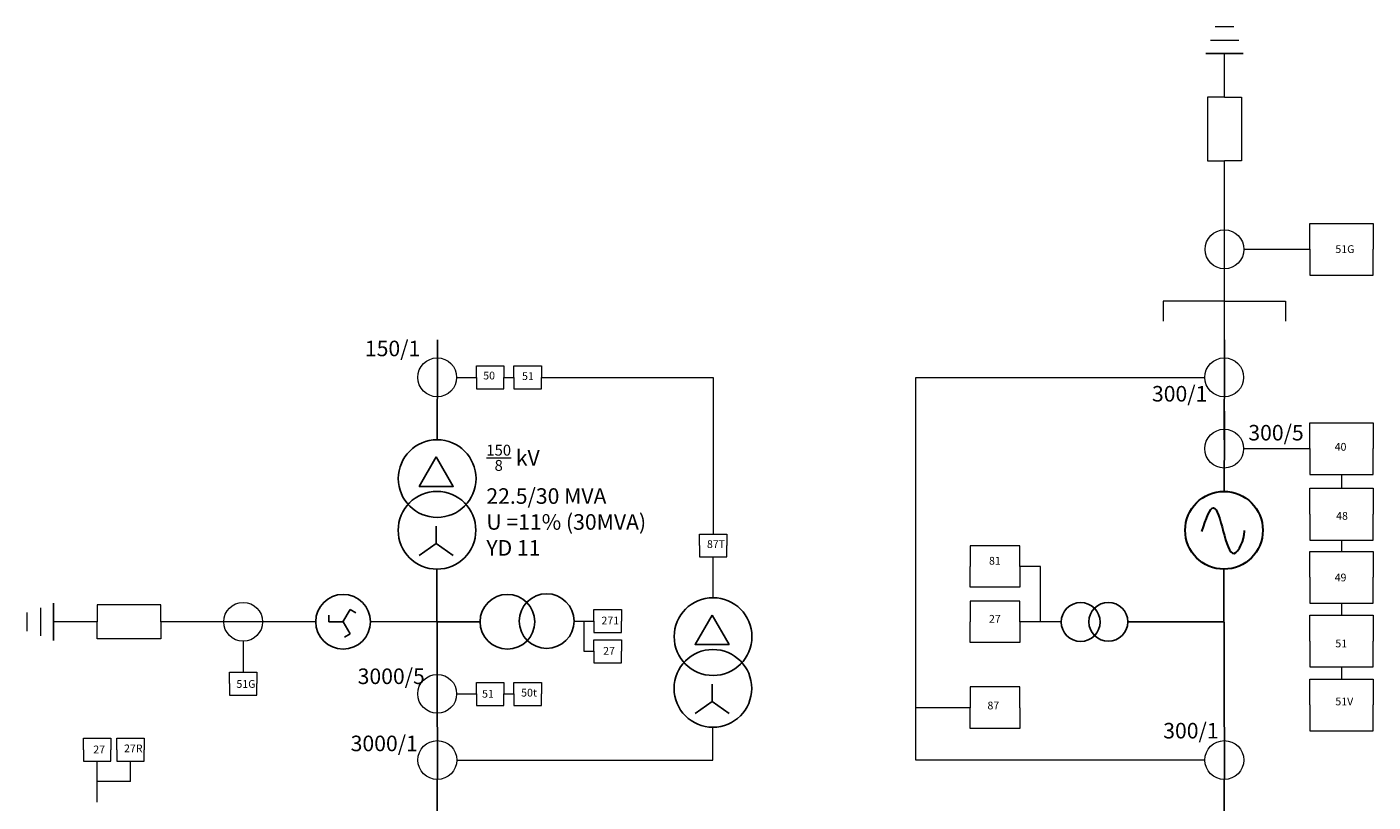
# Model space of a CAD drawing. Units: inches. Extents: x 77.1 to 95.7, y 45.4 to 81.6.
# Tile 3 of 3: x 78.4 to 95.7, y 71.6 to 81.6. Entities that reach past the tile are written whole.
import ezdxf

# ---------------------------------------------------------------- set-up
doc = ezdxf.new("R2010")
doc.units = ezdxf.units.IN
doc.header["$MEASUREMENT"] = 0
for name, color, linetype, lineweight in [('E-ANNO-TEXT', 7, 'Continuous', 18), ('E-POWR-CT', 4, 'Continuous', 18), ('E-POWR-EQPM', 3, 'Continuous', 30), ('E-POWR-FEED', 7, 'Continuous', 25), ('E-POWR-GRND', 3, 'Continuous', 18), ('E-POWR-XFMR', 4, 'Continuous', 25), ('E-PROT-RELY', 2, 'Continuous', 18), ('E-PROT-TEXT', 7, 'Continuous', 13), ('E-PROT-WIRE', 5, 'Continuous', 13)]:
    doc.layers.add(name, color=color, linetype=linetype, lineweight=lineweight)
doc.styles.get("Standard").update_dxf_attribs({"font": 'arial.ttf'})

# ---------------------------------------------------------------- blocks, each defined once
blk = doc.blocks.new('*U1')
for p, q in [((-0.091, -0.042), (-0.091, 0.042)), ((0.091, -0.042), (-0.091, -0.042))]:
    blk.add_line(p, q)
blk = doc.blocks.new('*U2')
at = {"layer": 'E-POWR-XFMR', "color": 0, "linetype": 'ByBlock', "lineweight": -2, "transparency": 16777216}
blk.add_blockref('*U1', (22.696, 22.881), dxfattribs=at)
for p, rotation in [((22.868, 22.897), 240), ((22.796, 22.74), 120)]:
    blk.add_blockref('*U1', p, dxfattribs=dict(at, rotation=rotation))
blk = doc.blocks.new('XFMR-DELTA-WYE')
for p, q in [((0.49, 0.555), (0.49, 0.332)), ((0.49, 0.332), (0.271, 0.175)), ((0.49, 0.332), (0.709, 0.175))]:
    blk.add_line(p, q)
blk.add_lwpolyline([(0.49, 1.444), (0.271, 1.065), (0.709, 1.065)], close=True)
for centre in [(0.502, 1.166), (0.5, 0.5)]:
    blk.add_circle(centre, 0.5)
blk = doc.blocks.new('CT-SINGLE')
blk.add_circle((0.25, 0.25), 0.25)
blk = doc.blocks.new('NEUTRAL-GROUNDING-RESISTOR')
for p, q in [((0.82, 0.438), (0, 0.438)), ((0, 0.438), (0, 0.219)), ((0.82, 0.219), (0.82, 0.438)), ((0, 0), (0, 0.219)), ((0.82, 0.219), (0.82, 0)), ((0.82, 0), (0, 0))]:
    blk.add_line(p, q)
blk = doc.blocks.new('EARTH-GROUND')
for p, q in [((0, 0.36), (0, 0.12)), ((0.174, 0.421), (0.174, 0.059))]:
    blk.add_line(p, q)
for points in [[(0.342, 0.24), (0.342, 0.24), (0.342, 0.48), (0.342, 0.48)], [(0.342, 0.24), (0.342, 0.24), (0.342, 0), (0.342, 0)]]:
    blk.add_lwpolyline(points, close=True)
blk = doc.blocks.new('RELAY-FUNCTION')
for p, q in [((0, 0.148), (0, 0.295)), ((0, 0.295), (0.353, 0.295)), ((0.353, 0.295), (0.353, 0.148)), ((0, 0.148), (0, 0)), ((0, 0), (0.353, 0)), ((0.353, 0), (0.353, 0.148))]:
    blk.add_line(p, q)
blk = doc.blocks.new('RELAY-FUNCTION-MED')
for p, q in [((0.638, 0.533), (0, 0.533)), ((0, 0.533), (0, 0.266)), ((0.638, 0.266), (0.638, 0.533)), ((0, 0), (0, 0.266)), ((0.638, 0.266), (0.638, 0)), ((0.638, 0), (0, 0))]:
    blk.add_line(p, q)
blk = doc.blocks.new('RELAY-FUNCTION-LARGE')
for p, q in [((0, 0.333), (0, 0.666)), ((0, 0.666), (0.813, 0.666)), ((0.813, 0.666), (0.813, 0.333)), ((0, 0.333), (0, 0)), ((0.813, 0), (0.813, 0.333)), ((0, 0), (0.813, 0))]:
    blk.add_line(p, q)

msp = doc.modelspace()

# ---------------------------------------------------------------- linework, layer by layer
at = {"layer": 'E-POWR-EQPM'}
msp.add_circle((93.785, 75.121), 0.5, dxfattribs=at)
msp.add_open_spline([(93.501, 75.107), (93.553, 75.261), (93.656, 75.563), (93.771, 75.115), (93.899, 74.667), (94.049, 75.007), (94.049, 75.114), (94.049, 75.117)], degree=3, knots=[0, 0, 0, 0, 0.339265, 0.667803, 0.983667, 1.296423, 1.305933, 1.305933, 1.305933, 1.305933], dxfattribs=at)
at = {"layer": 'E-POWR-FEED'}
for p, q in [((83.663, 77.339), (83.663, 77.572)), ((93.79, 77.339), (93.79, 77.572)), ((83.66, 76.287), (83.663, 77.339)), ((93.787, 76.287), (93.79, 77.339)), ((93.79, 76.422), (93.79, 76.656)), ((93.788, 75.621), (93.79, 76.422)), ((83.661, 73.267), (83.658, 74.621)), ((93.788, 73.267), (93.785, 74.621)), ((83.659, 73.944), (84.212, 73.944)), ((93.786, 73.944), (92.547, 73.944)), ((83.663, 71.915), (83.66, 73.267)), ((93.79, 71.915), (93.787, 73.267)), ((83.662, 71.105), (83.662, 71.915)), ((93.789, 71.105), (93.789, 71.915))]:
    msp.add_line(p, q, dxfattribs=at)
at = {"layer": 'E-POWR-GRND'}
for p, q in [((93.793, 80.695), (93.793, 81.256)), ((93.793, 79.22), (93.793, 79.875)), ((93.793, 78.987), (93.793, 79.22)), ((93.79, 77.934), (93.793, 78.987)), ((93.793, 78.07), (93.793, 78.303)), ((93.79, 78.07), (93.004, 78.07)), ((93.004, 78.07), (93.004, 77.811)), ((93.79, 77.572), (93.79, 78.07)), ((93.79, 78.07), (94.577, 78.07)), ((94.577, 78.07), (94.577, 77.811)), ((79.284, 73.944), (78.723, 73.944)), ((81.414, 73.944), (80.104, 73.944)), ((82.097, 73.944), (81.414, 73.944)), ((83.659, 73.944), (82.801, 73.944))]:
    msp.add_line(p, q, dxfattribs=at)
at = {"layer": 'E-POWR-XFMR'}
for centre, radius in [((82.449, 73.944), 0.352), ((84.564, 73.944), 0.352), ((85.069, 73.953), 0.352), ((91.941, 73.941), 0.25), ((92.297, 73.944), 0.25)]:
    msp.add_circle(centre, radius, dxfattribs=at)
at = {"layer": 'E-PROT-WIRE'}
for p, q in [((94.038, 78.737), (94.89, 78.737)), ((83.911, 77.089), (84.167, 77.089)), ((84.52, 77.089), (84.648, 77.089)), ((85.001, 77.089), (87.211, 77.089)), ((87.211, 77.089), (87.211, 75.074)), ((89.819, 72.165), (89.819, 77.089)), ((89.819, 77.089), (93.538, 77.089)), ((94.038, 76.172), (94.89, 76.172)), ((95.297, 75.839), (95.297, 75.662)), ((95.297, 74.996), (95.297, 74.85)), ((87.21, 74.253), (87.211, 74.779)), ((91.424, 74.655), (91.157, 74.655)), ((91.424, 73.944), (91.424, 74.655)), ((95.297, 74.184), (95.297, 74.028)), ((85.421, 73.953), (85.677, 73.953)), ((85.549, 73.953), (85.549, 73.564)), ((91.691, 73.944), (91.157, 73.944)), ((81.164, 73.694), (81.162, 73.296)), ((85.549, 73.564), (85.677, 73.564)), ((95.297, 73.363), (95.297, 73.207)), ((83.911, 73.017), (84.167, 73.017)), ((84.52, 73.017), (84.648, 73.017)), ((90.519, 72.839), (89.819, 72.839)), ((87.208, 72.165), (87.208, 72.587)), ((79.283, 71.624), (79.285, 72.15)), ((79.715, 71.887), (79.715, 72.15)), ((83.912, 72.165), (87.208, 72.165)), ((93.539, 72.165), (89.819, 72.165)), ((79.715, 71.887), (79.284, 71.887))]:
    msp.add_line(p, q, dxfattribs=at)

# ---------------------------------------------------------------- block references
at = {"layer": 'E-POWR-CT'}
for p in [(93.541, 78.486), (83.411, 76.839), (93.538, 76.839), (93.538, 75.922), (80.914, 73.694), (83.411, 72.767), (83.412, 71.915), (93.539, 71.915)]:
    msp.add_blockref('CT-SINGLE', p, dxfattribs=at)
at = {"layer": 'E-POWR-GRND'}
for name, p, rotation in [('EARTH-GROUND', (93.553, 81.598), 269.9999999999964), ('NEUTRAL-GROUNDING-RESISTOR', (94.012, 79.875), 89.99999999999834)]:
    msp.add_blockref(name, p, dxfattribs=dict(at, rotation=rotation))
for name, p in [('EARTH-GROUND', (78.381, 73.704)), ('NEUTRAL-GROUNDING-RESISTOR', (79.284, 73.725))]:
    msp.add_blockref(name, p, dxfattribs=at)
at = {"layer": 'E-POWR-XFMR'}
for name, p in [('XFMR-DELTA-WYE', (83.158, 74.621)), ('XFMR-DELTA-WYE', (86.708, 72.587)), ('*U2', (59.662, 51.105))]:
    msp.add_blockref(name, p, dxfattribs=at)
at = {"layer": 'E-PROT-RELY'}
for name, p in [('RELAY-FUNCTION-LARGE', (94.89, 78.404)), ('RELAY-FUNCTION', (84.167, 76.941)), ('RELAY-FUNCTION', (84.648, 76.941)), ('RELAY-FUNCTION-LARGE', (94.89, 75.839)), ('RELAY-FUNCTION-LARGE', (94.89, 74.996)), ('RELAY-FUNCTION', (87.035, 74.778)), ('RELAY-FUNCTION-MED', (90.519, 74.389)), ('RELAY-FUNCTION-LARGE', (94.89, 74.184)), ('RELAY-FUNCTION-MED', (90.519, 73.678)), ('RELAY-FUNCTION', (85.677, 73.805)), ('RELAY-FUNCTION-LARGE', (94.89, 73.363)), ('RELAY-FUNCTION', (85.677, 73.417)), ('RELAY-FUNCTION', (80.986, 73.001)), ('RELAY-FUNCTION', (84.167, 72.869)), ('RELAY-FUNCTION', (84.648, 72.869)), ('RELAY-FUNCTION-MED', (90.519, 72.573)), ('RELAY-FUNCTION-LARGE', (94.89, 72.541)), ('RELAY-FUNCTION', (79.108, 72.15)), ('RELAY-FUNCTION', (79.539, 72.15))]:
    msp.add_blockref(name, p, dxfattribs=at)

# ---------------------------------------------------------------- texts
at = {"layer": 'E-ANNO-TEXT', "char_height": 0.2, "attachment_point": 1}
for s, width, insert in [('150/1', 0.93095, (82.73, 77.561)), ('300/1', 0.93095, (92.858, 76.978)), ('300/5', 0.93095, (94.098, 76.477)), ('\\A1;{\\H0.7x;\\S150/8;} kV\\P22.5/30 MVA\\PU =11% (30MVA)\\PYD 11', 2.97281, (84.293, 76.222)), ('3000/5', 0.93095, (82.637, 73.343)), ('300/1', 0.93095, (93.003, 72.643)), ('3000/1', 0.93095, (82.547, 72.479))]:
    msp.add_mtext_dynamic_manual_height_columns(s, width=width, gutter_width=1, heights=[0], dxfattribs=dict(at, insert=insert))
at = {"layer": 'E-PROT-TEXT', "char_height": 0.1, "attachment_point": 1}
for s, width, heights, insert in [('51G', 0.27964, [0], (95.218, 78.789)), ('50', 0.27964, [0], (84.253, 77.162)), ('51', 0.27964, [0], (84.752, 77.155)), ('40', 0.27964, [0], (95.209, 76.245)), ('48', 0.27964, [0], (95.228, 75.357)), ('87T', 0.27964, [0], (87.132, 74.993)), ('81', 0.15659, [0.102], (90.761, 74.779)), ('49', 0.27964, [0], (95.209, 74.564)), ('271', 0.27964, [0], (85.774, 74.01)), ('27', 0.27964, [0], (90.761, 74.032)), ('27', 0.27964, [0], (85.796, 73.62)), ('51', 0.27964, [0], (95.218, 73.715)), ('51G', 0.27964, [0], (81.077, 73.194)), ('51', 0.27964, [0], (84.238, 73.068)), ('50t', 0.27964, [0], (84.741, 73.082)), ('51V', 0.27964, [0], (95.218, 72.969)), ('87', 0.27964, [0], (90.741, 72.917)), ('27', 0.27964, [0], (79.235, 72.351)), ('27R', 0.27964, [0], (79.631, 72.365))]:
    msp.add_mtext_dynamic_manual_height_columns(s, width=width, gutter_width=1, heights=heights, dxfattribs=dict(at, insert=insert))

doc.saveas('drawing.dxf')
